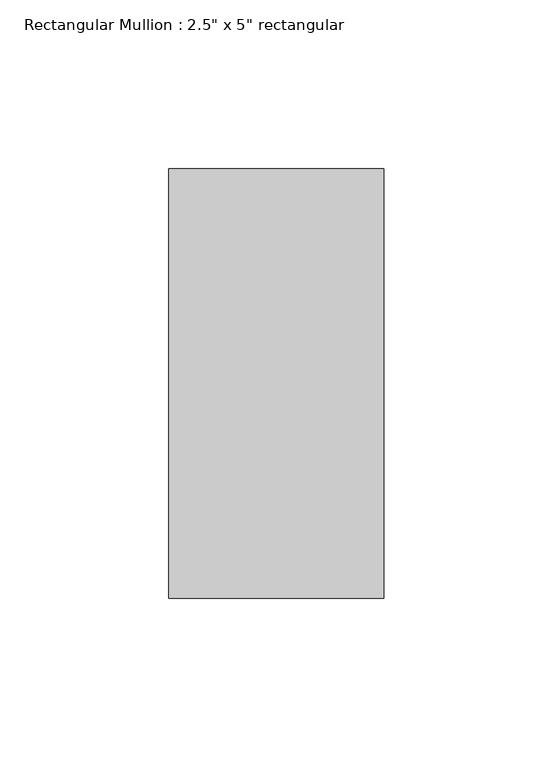
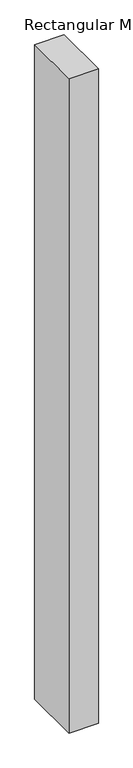
"""IFC4 building model written with IfcOpenShell, lengths in millimetres: member geometry."""

from ifc_helpers import new_model, si_unit, frame, origin, place, context, project, spatial, polyline, outline, extrude, source, transform, mapped, element, save


def member_75cd65a6(model_context):
    return source(origin(), model_context, "Body", "SweptSolid", [
        extrude(outline(polyline([(31.75, 63.5), (31.75, -63.5), (-31.75, -63.5), (-31.75, 63.5), (31.75, 63.5)])), frame((0.0, 0.0, -1486.9744191), z_axis=(0.0, 0.0, 1.0), x_axis=(1.0, 0.0, 0.0)), (0.0, 0.0, 1.0), 1486.9744191),
    ])


if __name__ == "__main__":
    model = new_model("IFC4")
    model_context = context("Model", 3, world=origin())
    ifc_project = project(units=[si_unit("LENGTHUNIT", "METRE", prefix="MILLI")], contexts=[model_context])
    site = spatial("IfcSite", under=ifc_project)
    building = spatial("IfcBuilding", under=site)
    placement = place(None, origin())
    member_shape = member_75cd65a6(model_context)
    element("IfcMember", 1, ObjectType="Rectangular Mullion : 2.5\" x 5\" rectangular", at=placement, inside=building, context=model_context, shape_type="MappedRepresentation", body=[
        mapped(member_shape, transform((0.0, 0.0, 0.0), x_axis=(1.0, 0.0, 0.0), y_axis=(0.0, 1.0, 0.0), z_axis=(0.0, 0.0, 1.0))),
    ])
    save(model, "model.ifc")

# Revit data of these elements
# Type "Rectangular Mullion : 2.5\" x 5\" rectangular"
#   built-in parameter 1007304 = 0.416667 (stored number, unit not read)
#   built-in parameter 1007301 = 0.104167 (stored number, unit not read)
#   built-in parameter 1007300 = 0.104167 (stored number, unit not read)
# Element 1 (IfcMember, "Rectangular Mullion : 2.5\" x 5\" rectangular")
#   Materials on its faces: "Aluminum"
# Materials
#   "Aluminum": class "Metal", colour RGB 247 247 247, transparency 0, Description = "Aluminum 6061", Cost = 0
